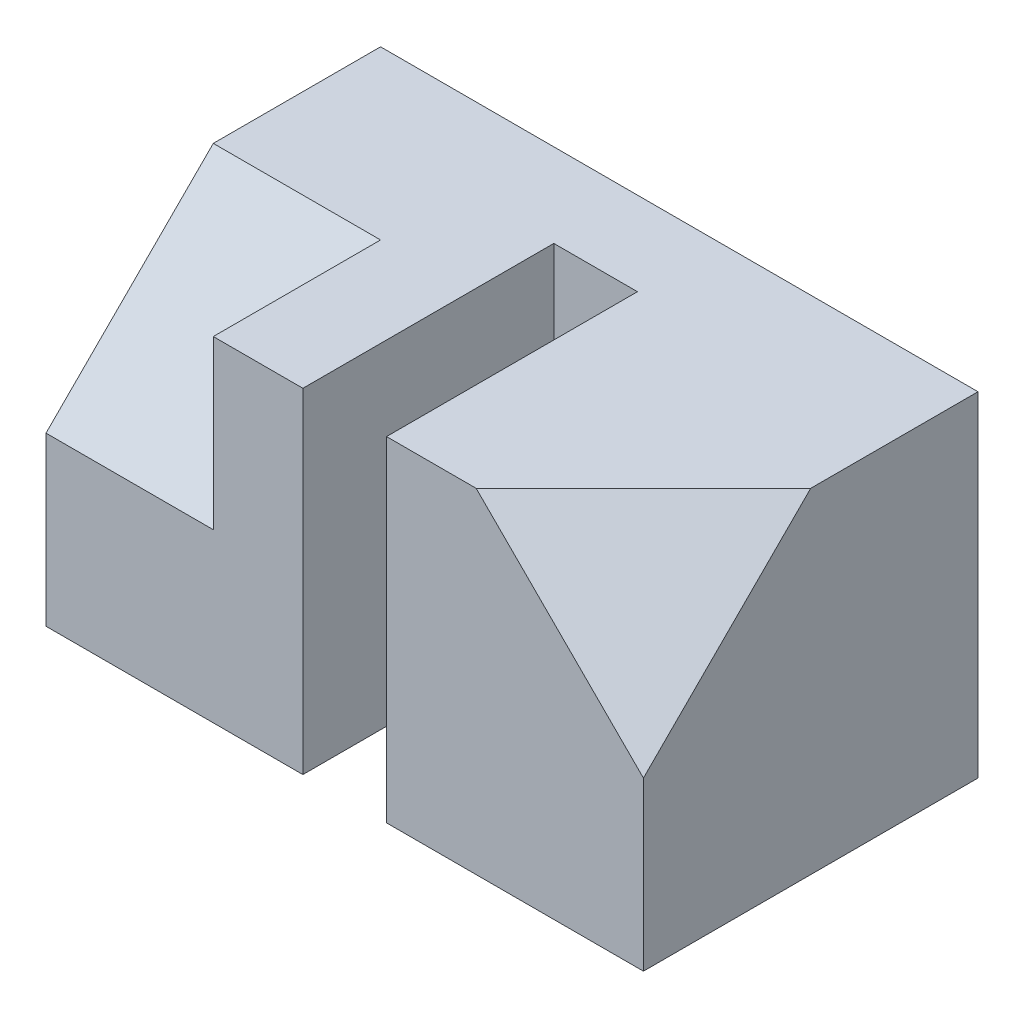
ISO-10303-21;
HEADER;
FILE_DESCRIPTION(('STEP AP214'),'2;1');
FILE_NAME('part.step','',(''),(''),'','','');
FILE_SCHEMA(('AUTOMOTIVE_DESIGN { 1 0 10303 214 1 1 1 1 }'));
ENDSEC;
DATA;
#1=APPLICATION_CONTEXT('core data for automotive mechanical design processes');
#2=APPLICATION_PROTOCOL_DEFINITION('international standard','automotive_design',2000,#1);
#3=PRODUCT_CONTEXT('',#1,'mechanical');
#4=PRODUCT('Part','Part','',(#3));
#5=PRODUCT_RELATED_PRODUCT_CATEGORY('part','',(#4));
#6=PRODUCT_DEFINITION_FORMATION('','',#4);
#7=PRODUCT_DEFINITION_CONTEXT('part definition',#1,'design');
#8=PRODUCT_DEFINITION('design','',#6,#7);
#9=PRODUCT_DEFINITION_SHAPE('','',#8);
#10=(LENGTH_UNIT() NAMED_UNIT(*) SI_UNIT(.MILLI.,.METRE.));
#11=(NAMED_UNIT(*) PLANE_ANGLE_UNIT() SI_UNIT($,.RADIAN.));
#12=(NAMED_UNIT(*) SI_UNIT($,.STERADIAN.) SOLID_ANGLE_UNIT());
#13=UNCERTAINTY_MEASURE_WITH_UNIT(LENGTH_MEASURE(1.E-05),#10,'distance_accuracy_value','');
#14=(GEOMETRIC_REPRESENTATION_CONTEXT(3) GLOBAL_UNCERTAINTY_ASSIGNED_CONTEXT((#13)) GLOBAL_UNIT_ASSIGNED_CONTEXT((#10,
#11,#12)) REPRESENTATION_CONTEXT('',''));
#15=CARTESIAN_POINT('',(0.,0.,0.));
#16=DIRECTION('',(0.,0.,1.));
#17=DIRECTION('',(1.,0.,0.));
#18=AXIS2_PLACEMENT_3D('',#15,#16,#17);
#19=CARTESIAN_POINT('',(0.,28.,0.));
#20=DIRECTION('',(0.,1.,0.));
#21=DIRECTION('',(0.,0.,1.));
#22=AXIS2_PLACEMENT_3D('',#19,#20,#21);
#23=PLANE('',#22);
#24=DIRECTION('',(1.,0.,0.));
#25=VECTOR('',#24,1.);
#26=CARTESIAN_POINT('',(-25.,28.,14.));
#27=LINE('',#26,#25);
#28=CARTESIAN_POINT('',(3.5,28.,14.));
#29=VERTEX_POINT('',#28);
#30=CARTESIAN_POINT('',(11.,28.,14.));
#31=VERTEX_POINT('',#30);
#32=EDGE_CURVE('E132',#29,#31,#27,.T.);
#33=ORIENTED_EDGE('',*,*,#32,.T.);
#34=DIRECTION('',(0.707106781186547,0.,-0.707106781186548));
#35=VECTOR('',#34,1.);
#36=CARTESIAN_POINT('',(12.5,28.,12.5));
#37=LINE('',#36,#35);
#38=CARTESIAN_POINT('',(25.,28.,0.));
#39=VERTEX_POINT('',#38);
#40=EDGE_CURVE('E11',#31,#39,#37,.T.);
#41=ORIENTED_EDGE('',*,*,#40,.T.);
#42=DIRECTION('',(0.,0.,-1.));
#43=VECTOR('',#42,1.);
#44=CARTESIAN_POINT('',(25.,28.,-14.));
#45=LINE('',#44,#43);
#46=CARTESIAN_POINT('',(25.,28.,-14.));
#47=VERTEX_POINT('',#46);
#48=EDGE_CURVE('E159',#39,#47,#45,.T.);
#49=ORIENTED_EDGE('',*,*,#48,.T.);
#50=DIRECTION('',(-1.,0.,0.));
#51=VECTOR('',#50,1.);
#52=CARTESIAN_POINT('',(-25.,28.,-14.));
#53=LINE('',#52,#51);
#54=CARTESIAN_POINT('',(-25.,28.,-14.));
#55=VERTEX_POINT('',#54);
#56=EDGE_CURVE('E141',#47,#55,#53,.T.);
#57=ORIENTED_EDGE('',*,*,#56,.T.);
#58=DIRECTION('',(0.,0.,1.));
#59=VECTOR('',#58,1.);
#60=CARTESIAN_POINT('',(-25.,28.,-14.));
#61=LINE('',#60,#59);
#62=CARTESIAN_POINT('',(-25.,28.,0.));
#63=VERTEX_POINT('',#62);
#64=EDGE_CURVE('E139',#55,#63,#61,.T.);
#65=ORIENTED_EDGE('',*,*,#64,.T.);
#66=DIRECTION('',(-1.,0.,0.));
#67=VECTOR('',#66,1.);
#68=CARTESIAN_POINT('',(-11.,28.,0.));
#69=LINE('',#68,#67);
#70=CARTESIAN_POINT('',(-11.,28.,0.));
#71=VERTEX_POINT('',#70);
#72=EDGE_CURVE('E195',#71,#63,#69,.T.);
#73=ORIENTED_EDGE('',*,*,#72,.F.);
#74=DIRECTION('',(0.,0.,-1.));
#75=VECTOR('',#74,1.);
#76=CARTESIAN_POINT('',(-11.,28.,0.));
#77=LINE('',#76,#75);
#78=CARTESIAN_POINT('',(-11.,28.,14.));
#79=VERTEX_POINT('',#78);
#80=EDGE_CURVE('E222',#79,#71,#77,.T.);
#81=ORIENTED_EDGE('',*,*,#80,.F.);
#82=CARTESIAN_POINT('',(-3.5,28.,14.));
#83=VERTEX_POINT('',#82);
#84=EDGE_CURVE('E138',#79,#83,#27,.T.);
#85=ORIENTED_EDGE('',*,*,#84,.T.);
#86=DIRECTION('',(0.,0.,1.));
#87=VECTOR('',#86,1.);
#88=CARTESIAN_POINT('',(-3.5,28.,-7.));
#89=LINE('',#88,#87);
#90=CARTESIAN_POINT('',(-3.5,28.,-7.));
#91=VERTEX_POINT('',#90);
#92=EDGE_CURVE('E207',#91,#83,#89,.T.);
#93=ORIENTED_EDGE('',*,*,#92,.F.);
#94=DIRECTION('',(-1.,0.,0.));
#95=VECTOR('',#94,1.);
#96=CARTESIAN_POINT('',(-3.5,28.,-7.));
#97=LINE('',#96,#95);
#98=CARTESIAN_POINT('',(3.5,28.,-7.));
#99=VERTEX_POINT('',#98);
#100=EDGE_CURVE('E204',#99,#91,#97,.T.);
#101=ORIENTED_EDGE('',*,*,#100,.F.);
#102=DIRECTION('',(0.,0.,-1.));
#103=VECTOR('',#102,1.);
#104=CARTESIAN_POINT('',(3.5,28.,-7.));
#105=LINE('',#104,#103);
#106=EDGE_CURVE('E137',#29,#99,#105,.T.);
#107=ORIENTED_EDGE('',*,*,#106,.F.);
#108=EDGE_LOOP('',(#33,#41,#49,#57,#65,#73,#81,#85,#93,#101,#107));
#109=FACE_BOUND('',#108,.T.);
#110=ADVANCED_FACE('F41',(#109),#23,.T.);
#111=CARTESIAN_POINT('',(-25.,28.,14.));
#112=DIRECTION('',(0.,0.,-1.));
#113=DIRECTION('',(-1.,0.,0.));
#114=AXIS2_PLACEMENT_3D('',#111,#112,#113);
#115=PLANE('',#114);
#116=DIRECTION('',(0.,1.,0.));
#117=VECTOR('',#116,1.);
#118=CARTESIAN_POINT('',(-11.,28.,14.));
#119=LINE('',#118,#117);
#120=CARTESIAN_POINT('',(-11.,14.,14.));
#121=VERTEX_POINT('',#120);
#122=EDGE_CURVE('E64',#121,#79,#119,.T.);
#123=ORIENTED_EDGE('',*,*,#122,.F.);
#124=DIRECTION('',(-1.,0.,0.));
#125=VECTOR('',#124,1.);
#126=CARTESIAN_POINT('',(-11.,14.,14.));
#127=LINE('',#126,#125);
#128=CARTESIAN_POINT('',(-25.,14.,14.));
#129=VERTEX_POINT('',#128);
#130=EDGE_CURVE('E215',#121,#129,#127,.T.);
#131=ORIENTED_EDGE('',*,*,#130,.T.);
#132=DIRECTION('',(0.,-1.,0.));
#133=VECTOR('',#132,1.);
#134=CARTESIAN_POINT('',(-25.,28.,14.));
#135=LINE('',#134,#133);
#136=CARTESIAN_POINT('',(-25.,0.,14.));
#137=VERTEX_POINT('',#136);
#138=EDGE_CURVE('E165',#129,#137,#135,.T.);
#139=ORIENTED_EDGE('',*,*,#138,.T.);
#140=DIRECTION('',(1.,0.,0.));
#141=VECTOR('',#140,1.);
#142=CARTESIAN_POINT('',(-25.,0.,14.));
#143=LINE('',#142,#141);
#144=CARTESIAN_POINT('',(-3.5,0.,14.));
#145=VERTEX_POINT('',#144);
#146=EDGE_CURVE('E160',#137,#145,#143,.T.);
#147=ORIENTED_EDGE('',*,*,#146,.T.);
#148=DIRECTION('',(0.,1.,0.));
#149=VECTOR('',#148,1.);
#150=CARTESIAN_POINT('',(-3.5,0.,14.));
#151=LINE('',#150,#149);
#152=EDGE_CURVE('E194',#145,#83,#151,.T.);
#153=ORIENTED_EDGE('',*,*,#152,.T.);
#154=ORIENTED_EDGE('',*,*,#84,.F.);
#155=EDGE_LOOP('',(#123,#131,#139,#147,#153,#154));
#156=FACE_BOUND('',#155,.T.);
#157=ADVANCED_FACE('F228',(#156),#115,.F.);
#158=CARTESIAN_POINT('',(25.,28.,-14.));
#159=DIRECTION('',(-1.,0.,0.));
#160=DIRECTION('',(0.,0.,1.));
#161=AXIS2_PLACEMENT_3D('',#158,#159,#160);
#162=PLANE('',#161);
#163=DIRECTION('',(0.,0.707106781186548,-0.707106781186548));
#164=VECTOR('',#163,1.);
#165=CARTESIAN_POINT('',(25.,35.,-6.99999999999999));
#166=LINE('',#165,#164);
#167=CARTESIAN_POINT('',(25.,14.,14.));
#168=VERTEX_POINT('',#167);
#169=EDGE_CURVE('E57',#168,#39,#166,.T.);
#170=ORIENTED_EDGE('',*,*,#169,.F.);
#171=DIRECTION('',(0.,-1.,0.));
#172=VECTOR('',#171,1.);
#173=CARTESIAN_POINT('',(25.,28.,14.));
#174=LINE('',#173,#172);
#175=CARTESIAN_POINT('',(25.,0.,14.));
#176=VERTEX_POINT('',#175);
#177=EDGE_CURVE('E133',#168,#176,#174,.T.);
#178=ORIENTED_EDGE('',*,*,#177,.T.);
#179=DIRECTION('',(0.,0.,-1.));
#180=VECTOR('',#179,1.);
#181=CARTESIAN_POINT('',(25.,0.,-14.));
#182=LINE('',#181,#180);
#183=CARTESIAN_POINT('',(25.,0.,-14.));
#184=VERTEX_POINT('',#183);
#185=EDGE_CURVE('E150',#176,#184,#182,.T.);
#186=ORIENTED_EDGE('',*,*,#185,.T.);
#187=DIRECTION('',(0.,-1.,0.));
#188=VECTOR('',#187,1.);
#189=CARTESIAN_POINT('',(25.,28.,-14.));
#190=LINE('',#189,#188);
#191=EDGE_CURVE('E170',#47,#184,#190,.T.);
#192=ORIENTED_EDGE('',*,*,#191,.F.);
#193=ORIENTED_EDGE('',*,*,#48,.F.);
#194=EDGE_LOOP('',(#170,#178,#186,#192,#193));
#195=FACE_BOUND('',#194,.T.);
#196=ADVANCED_FACE('F43',(#195),#162,.F.);
#197=CARTESIAN_POINT('',(-25.,28.,-14.));
#198=DIRECTION('',(0.,0.,1.));
#199=DIRECTION('',(1.,0.,0.));
#200=AXIS2_PLACEMENT_3D('',#197,#198,#199);
#201=PLANE('',#200);
#202=DIRECTION('',(-1.,0.,0.));
#203=VECTOR('',#202,1.);
#204=CARTESIAN_POINT('',(-25.,0.,-14.));
#205=LINE('',#204,#203);
#206=CARTESIAN_POINT('',(-25.,0.,-14.));
#207=VERTEX_POINT('',#206);
#208=EDGE_CURVE('E147',#184,#207,#205,.T.);
#209=ORIENTED_EDGE('',*,*,#208,.T.);
#210=DIRECTION('',(0.,-1.,0.));
#211=VECTOR('',#210,1.);
#212=CARTESIAN_POINT('',(-25.,28.,-14.));
#213=LINE('',#212,#211);
#214=EDGE_CURVE('E163',#55,#207,#213,.T.);
#215=ORIENTED_EDGE('',*,*,#214,.F.);
#216=ORIENTED_EDGE('',*,*,#56,.F.);
#217=ORIENTED_EDGE('',*,*,#191,.T.);
#218=EDGE_LOOP('',(#209,#215,#216,#217));
#219=FACE_BOUND('',#218,.T.);
#220=ADVANCED_FACE('F174',(#219),#201,.F.);
#221=CARTESIAN_POINT('',(-25.,28.,-14.));
#222=DIRECTION('',(1.,0.,0.));
#223=DIRECTION('',(0.,0.,-1.));
#224=AXIS2_PLACEMENT_3D('',#221,#222,#223);
#225=PLANE('',#224);
#226=ORIENTED_EDGE('',*,*,#138,.F.);
#227=DIRECTION('',(0.,-0.707106781186547,0.707106781186547));
#228=VECTOR('',#227,1.);
#229=CARTESIAN_POINT('',(-25.,14.,14.));
#230=LINE('',#229,#228);
#231=EDGE_CURVE('E190',#63,#129,#230,.T.);
#232=ORIENTED_EDGE('',*,*,#231,.F.);
#233=ORIENTED_EDGE('',*,*,#64,.F.);
#234=ORIENTED_EDGE('',*,*,#214,.T.);
#235=DIRECTION('',(0.,0.,1.));
#236=VECTOR('',#235,1.);
#237=CARTESIAN_POINT('',(-25.,0.,-14.));
#238=LINE('',#237,#236);
#239=EDGE_CURVE('E153',#207,#137,#238,.T.);
#240=ORIENTED_EDGE('',*,*,#239,.T.);
#241=EDGE_LOOP('',(#226,#232,#233,#234,#240));
#242=FACE_BOUND('',#241,.T.);
#243=ADVANCED_FACE('F187',(#242),#225,.F.);
#244=DIRECTION('',(0.707106781186548,-0.707106781186548,0.));
#245=VECTOR('',#244,1.);
#246=CARTESIAN_POINT('',(-7.,46.,14.));
#247=LINE('',#246,#245);
#248=EDGE_CURVE('E47',#31,#168,#247,.T.);
#249=ORIENTED_EDGE('',*,*,#248,.F.);
#250=ORIENTED_EDGE('',*,*,#32,.F.);
#251=DIRECTION('',(0.,1.,0.));
#252=VECTOR('',#251,1.);
#253=CARTESIAN_POINT('',(3.5,0.,14.));
#254=LINE('',#253,#252);
#255=CARTESIAN_POINT('',(3.5,0.,14.));
#256=VERTEX_POINT('',#255);
#257=EDGE_CURVE('E196',#256,#29,#254,.T.);
#258=ORIENTED_EDGE('',*,*,#257,.F.);
#259=EDGE_CURVE('E156',#256,#176,#143,.T.);
#260=ORIENTED_EDGE('',*,*,#259,.T.);
#261=ORIENTED_EDGE('',*,*,#177,.F.);
#262=EDGE_LOOP('',(#249,#250,#258,#260,#261));
#263=FACE_BOUND('',#262,.T.);
#264=ADVANCED_FACE('F128',(#263),#115,.F.);
#265=CARTESIAN_POINT('',(0.,0.,0.));
#266=DIRECTION('',(0.,1.,0.));
#267=DIRECTION('',(0.,0.,1.));
#268=AXIS2_PLACEMENT_3D('',#265,#266,#267);
#269=PLANE('',#268);
#270=DIRECTION('',(-1.,0.,0.));
#271=VECTOR('',#270,1.);
#272=CARTESIAN_POINT('',(-3.5,0.,-7.));
#273=LINE('',#272,#271);
#274=CARTESIAN_POINT('',(3.5,0.,-7.));
#275=VERTEX_POINT('',#274);
#276=CARTESIAN_POINT('',(-3.5,0.,-7.));
#277=VERTEX_POINT('',#276);
#278=EDGE_CURVE('E200',#275,#277,#273,.T.);
#279=ORIENTED_EDGE('',*,*,#278,.T.);
#280=DIRECTION('',(0.,0.,1.));
#281=VECTOR('',#280,1.);
#282=CARTESIAN_POINT('',(-3.5,0.,-7.));
#283=LINE('',#282,#281);
#284=EDGE_CURVE('E210',#277,#145,#283,.T.);
#285=ORIENTED_EDGE('',*,*,#284,.T.);
#286=ORIENTED_EDGE('',*,*,#146,.F.);
#287=ORIENTED_EDGE('',*,*,#239,.F.);
#288=ORIENTED_EDGE('',*,*,#208,.F.);
#289=ORIENTED_EDGE('',*,*,#185,.F.);
#290=ORIENTED_EDGE('',*,*,#259,.F.);
#291=DIRECTION('',(0.,0.,-1.));
#292=VECTOR('',#291,1.);
#293=CARTESIAN_POINT('',(3.5,0.,-7.));
#294=LINE('',#293,#292);
#295=EDGE_CURVE('E212',#256,#275,#294,.T.);
#296=ORIENTED_EDGE('',*,*,#295,.T.);
#297=EDGE_LOOP('',(#279,#285,#286,#287,#288,#289,#290,#296));
#298=FACE_BOUND('',#297,.T.);
#299=ADVANCED_FACE('F179',(#298),#269,.F.);
#300=CARTESIAN_POINT('',(-3.5,0.,-7.));
#301=DIRECTION('',(-1.,0.,0.));
#302=DIRECTION('',(0.,0.,1.));
#303=AXIS2_PLACEMENT_3D('',#300,#301,#302);
#304=PLANE('',#303);
#305=ORIENTED_EDGE('',*,*,#92,.T.);
#306=ORIENTED_EDGE('',*,*,#152,.F.);
#307=ORIENTED_EDGE('',*,*,#284,.F.);
#308=DIRECTION('',(0.,1.,0.));
#309=VECTOR('',#308,1.);
#310=CARTESIAN_POINT('',(-3.5,0.,-7.));
#311=LINE('',#310,#309);
#312=EDGE_CURVE('E151',#277,#91,#311,.T.);
#313=ORIENTED_EDGE('',*,*,#312,.T.);
#314=EDGE_LOOP('',(#305,#306,#307,#313));
#315=FACE_BOUND('',#314,.T.);
#316=ADVANCED_FACE('F235',(#315),#304,.F.);
#317=CARTESIAN_POINT('',(-3.5,0.,-7.));
#318=DIRECTION('',(0.,0.,-1.));
#319=DIRECTION('',(-1.,0.,0.));
#320=AXIS2_PLACEMENT_3D('',#317,#318,#319);
#321=PLANE('',#320);
#322=ORIENTED_EDGE('',*,*,#100,.T.);
#323=ORIENTED_EDGE('',*,*,#312,.F.);
#324=ORIENTED_EDGE('',*,*,#278,.F.);
#325=DIRECTION('',(0.,1.,0.));
#326=VECTOR('',#325,1.);
#327=CARTESIAN_POINT('',(3.5,0.,-7.));
#328=LINE('',#327,#326);
#329=EDGE_CURVE('E203',#275,#99,#328,.T.);
#330=ORIENTED_EDGE('',*,*,#329,.T.);
#331=EDGE_LOOP('',(#322,#323,#324,#330));
#332=FACE_BOUND('',#331,.T.);
#333=ADVANCED_FACE('F234',(#332),#321,.F.);
#334=CARTESIAN_POINT('',(3.5,0.,-7.));
#335=DIRECTION('',(1.,0.,0.));
#336=DIRECTION('',(0.,0.,-1.));
#337=AXIS2_PLACEMENT_3D('',#334,#335,#336);
#338=PLANE('',#337);
#339=ORIENTED_EDGE('',*,*,#106,.T.);
#340=ORIENTED_EDGE('',*,*,#329,.F.);
#341=ORIENTED_EDGE('',*,*,#295,.F.);
#342=ORIENTED_EDGE('',*,*,#257,.T.);
#343=EDGE_LOOP('',(#339,#340,#341,#342));
#344=FACE_BOUND('',#343,.T.);
#345=ADVANCED_FACE('F240',(#344),#338,.F.);
#346=CARTESIAN_POINT('',(-11.,14.,14.));
#347=DIRECTION('',(0.,-0.707106781186548,-0.707106781186548));
#348=DIRECTION('',(0.,0.707106781186548,-0.707106781186548));
#349=AXIS2_PLACEMENT_3D('',#346,#347,#348);
#350=PLANE('',#349);
#351=ORIENTED_EDGE('',*,*,#231,.T.);
#352=ORIENTED_EDGE('',*,*,#130,.F.);
#353=DIRECTION('',(0.,-0.707106781186547,0.707106781186547));
#354=VECTOR('',#353,1.);
#355=CARTESIAN_POINT('',(-11.,14.,14.));
#356=LINE('',#355,#354);
#357=EDGE_CURVE('E224',#71,#121,#356,.T.);
#358=ORIENTED_EDGE('',*,*,#357,.F.);
#359=ORIENTED_EDGE('',*,*,#72,.T.);
#360=EDGE_LOOP('',(#351,#352,#358,#359));
#361=FACE_BOUND('',#360,.T.);
#362=ADVANCED_FACE('F239',(#361),#350,.F.);
#363=CARTESIAN_POINT('',(-11.,0.,0.));
#364=DIRECTION('',(1.,0.,0.));
#365=DIRECTION('',(0.,0.,-1.));
#366=AXIS2_PLACEMENT_3D('',#363,#364,#365);
#367=PLANE('',#366);
#368=ORIENTED_EDGE('',*,*,#80,.T.);
#369=ORIENTED_EDGE('',*,*,#357,.T.);
#370=ORIENTED_EDGE('',*,*,#122,.T.);
#371=EDGE_LOOP('',(#368,#369,#370));
#372=FACE_BOUND('',#371,.T.);
#373=ADVANCED_FACE('F223',(#372),#367,.F.);
#374=CARTESIAN_POINT('',(17.6666666666667,17.6666666666667,17.6666666666667));
#375=DIRECTION('',(0.577350269189626,0.577350269189626,0.577350269189626));
#376=DIRECTION('',(-0.707106781186548,0.707106781186548,0.));
#377=AXIS2_PLACEMENT_3D('',#374,#375,#376);
#378=PLANE('',#377);
#379=ORIENTED_EDGE('',*,*,#248,.T.);
#380=ORIENTED_EDGE('',*,*,#169,.T.);
#381=ORIENTED_EDGE('',*,*,#40,.F.);
#382=EDGE_LOOP('',(#379,#380,#381));
#383=FACE_BOUND('',#382,.T.);
#384=ADVANCED_FACE('F122',(#383),#378,.T.);
#385=CLOSED_SHELL('',(#110,#157,#196,#220,#243,#264,#299,#316,#333,#345,#362,#373,#384));
#386=MANIFOLD_SOLID_BREP('B2',#385);
#387=ADVANCED_BREP_SHAPE_REPRESENTATION('',(#18,#386),#14);
#388=SHAPE_DEFINITION_REPRESENTATION(#9,#387);
ENDSEC;
END-ISO-10303-21;
